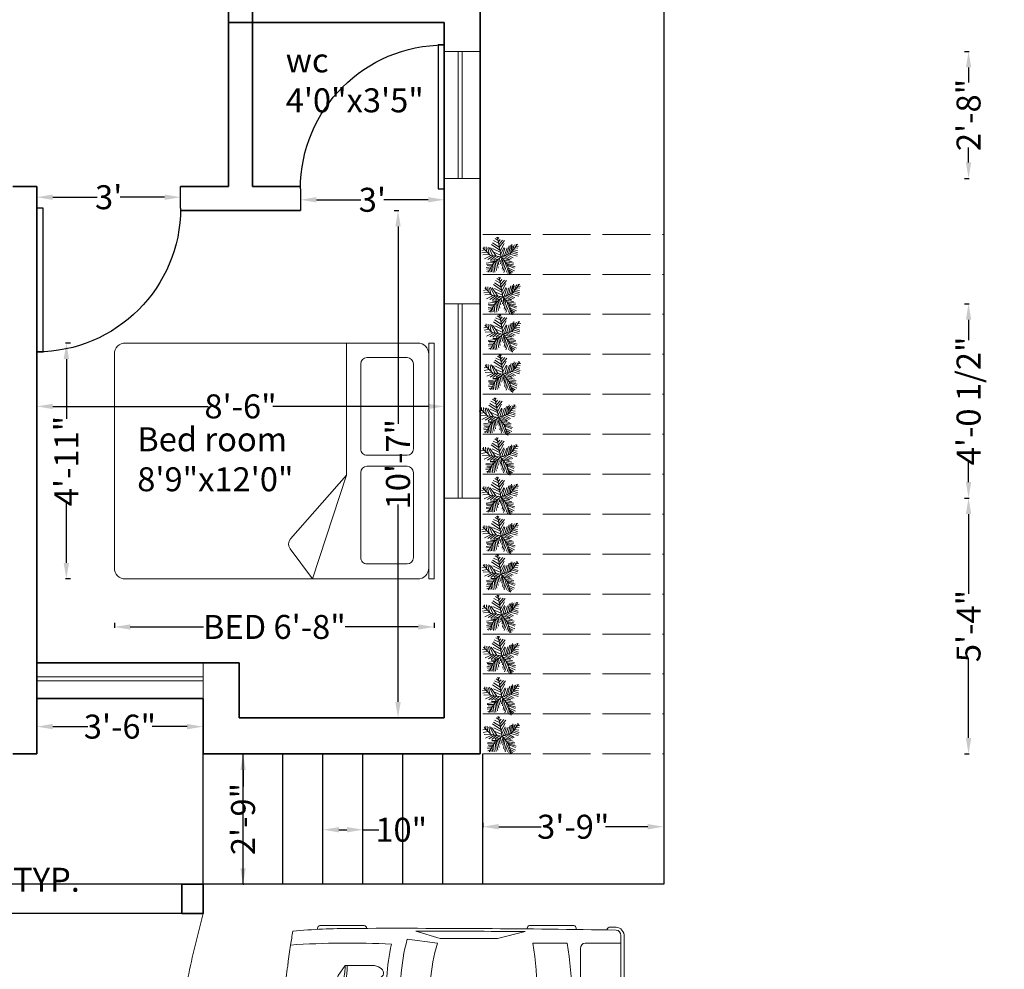
# Model space of a CAD drawing. Units: inches. Extents: x -81 to 380, y -521 to 79.
# Tile 4 of 5: x 134 to 380, y -313 to -76. Entities that reach past the tile are written whole.
import ezdxf

# ---------------------------------------------------------------- set-up
doc = ezdxf.new("R2010")
doc.units = ezdxf.units.IN
doc.header["$MEASUREMENT"] = 0
doc.linetypes.add('ACAD_ISO02W100', pattern=[15, 12, -3])
for name, color, linetype, lineweight in [('A-ANNO-DIMS', 2, 'Continuous', 18), ('A-AREA-IDEN', 5, 'Continuous', 25), ('A-COLS', 34, 'Continuous', 35), ('A-FLOR', 6, 'Continuous', 25), ('A-FLOR-STRS', 6, 'Continuous', 25), ('A-FLOR-STRS-OVHD', 6, 'ACAD_ISO02W100', 18), ('A-FURN', 8, 'Continuous', 18), ('A-GLAZ', 4, 'Continuous', 18), ('A-WALL', 249, 'Continuous', 35), ('C-ROAD-DRWY', 6, 'Continuous', 18), ('car', 33, 'Continuous', 18), ('door', 34, 'Continuous', 25), ('trees', 3, 'Continuous', 13)]:
    doc.layers.add(name, color=color, linetype=linetype, lineweight=lineweight)
doc.styles.get("Standard").update_dxf_attribs({"font": 'arial.ttf'})
doc.dimstyles.get("Standard").update_dxf_attribs({"dimtxt": 6, "dimasz": 4, "dimexe": 0.18, "dimexo": 0.0625, "dimgap": 0.09, "dimtad": 0, "dimdec": 0, "dimzin": 0, "dimdsep": 46, "dimlunit": 3, "dimtxsty": 'Standard', "dimcen": 0.09, "dimclrd": 6, "dimclre": 6, "dimclrt": 2, "dimadec": 0, "dimazin": 0, "dimtfac": 1, "dimtdec": 0, "dimtofl": 0, "dimtmove": 0, "dimatfit": 3, "dimfxl": 1, "dimfxlon": 1, "dimtolj": 1, "dimtzin": 0, "dimarcsym": 0})

# ---------------------------------------------------------------- blocks, each defined once
blk = doc.blocks.new('*U2')
for p, q in [((0, 0), (0, -6)), ((40, 0), (40, -6))]:
    blk.add_line(p, q)
blk.add_lwpolyline([(0, 0), (0, 40), (1.75, 40), (1.75, 0)], close=True)
blk.add_arc((0, 0), 40, 0, 90)
blk = doc.blocks.new('*U4')
for p, q in [((-48.585, 21.131), (-49.309, 29.026)), ((-43.513, 28.561), (-42.427, 15.558)), ((-3.665, 19.273), (-27.574, 35.527)), ((-5.114, 28.097), (-24.676, 40.636)), ((-7.288, 39.707), (-21.778, 46.673)), ((-8.737, 47.138), (-17.069, 52.711)), ((-10.186, 53.64), (-13.084, 55.962)), ((0, 0), (-10.5, 57)), ((-9.099, 51.782), (-6.563, 55.962)), ((-7.65, 43.423), (-2.578, 49.46)), ((-5.839, 35.992), (4.667, 48.067)), ((-5.114, 27.632), (10.463, 46.673)), ((-2.941, 16.486), (8.652, 37.85)), ((16.259, 5.805), (23.142, 31.348)), ((22.055, 7.198), (27.489, 32.277)), ((27, 9), (48, 36)), ((27.127, 9.056), (31.112, 35.992)), ((31.836, 30.883), (32.561, 16.486)), ((35.096, 32.741), (37.27, 22.524)), ((38.719, 34.134), (41.979, 28.561)), ((43.791, 29.954), (51.036, 30.883)), ((44.153, 36.456), (45.239, 32.741)), ((-47.498, 19.737), (-55.83, 18.344)), ((-40.615, 13.7), (-55.105, 10.913)), ((-31.5, 4.5), (-52.5, 25.5)), ((-33.37, 6.269), (-52.207, 5.34)), ((-28.299, 3.483), (-47.86, -5.805)), ((-38.442, 26.239), (-34.819, 7.663)), ((-21.416, 3.018), (-38.079, -8.128)), ((-35.544, 28.097), (-24.314, 3.947)), ((0, 0), (-31.5, 4.5)), ((-14.533, 2.09), (-30.834, 25.31)), ((-15.982, 2.09), (-30.11, -9.521)), ((-24.314, 23.917), (-2.941, 13.7)), ((0, 0), (-22.5, -19.5)), ((-6.563, 1.161), (-21.416, -8.128)), ((-20.691, 13.7), (-1.129, 4.876)), ((-1.129, 6.734), (9.014, 26.704)), ((0, 0), (27, 9)), ((0, 0), (18, -22.5)), ((3.942, 1.625), (11.187, 24.381)), ((6.478, 1.625), (26.04, -8.592)), ((10.101, 3.483), (17.708, 26.239)), ((11.187, 3.483), (30.749, -5.805)), ((18.07, 5.805), (35.096, -3.483)), ((24.229, 7.663), (46.688, 1.625)), ((29.662, 12.307), (48.137, 6.269)), ((33.285, 16.486), (48.862, 10.913)), ((36.183, 19.737), (48.137, 17.88)), ((40.53, 25.775), (48.862, 24.846)), ((-17.431, -15.094), (-42.789, -18.809)), ((-24.314, -21.596), (-42.427, -22.06)), ((-26.849, -26.24), (-40.253, -25.775)), ((-22.5, -19.5), (-37.5, -45)), ((-15.257, -12.772), (-30.11, -12.772)), ((-25.038, -23.918), (-22.865, -45.281)), ((-20.691, -18.345), (-17.793, -44.352)), ((-6.563, -5.805), (-19.967, -9.985)), ((-17.069, -15.094), (-12.721, -40.172)), ((-13.446, -11.378), (-8.737, -32.741)), ((-9.461, -8.592), (-6.201, -23.453)), ((-4.752, -3.483), (-3.665, -14.629)), ((2.493, -3.019), (-1.491, -20.202)), ((1.769, -2.555), (24.229, -9.521)), ((5.029, -6.27), (2.131, -25.775)), ((9.014, -11.378), (3.58, -35.992)), ((14.085, -16.951), (6.478, -40.172)), ((7.565, -9.056), (32.198, -14.629)), ((18.07, -22.524), (8.289, -45.745)), ((12.274, -15.094), (36.907, -18.809)), ((16.259, -19.738), (36.183, -22.989)), ((18, -22.5), (27, -52.5)), ((18.433, -22.524), (40.53, -29.026)), ((19.157, -25.311), (38.719, -33.206)), ((-28.299, -29.026), (-42.789, -31.348)), ((-30.834, -34.135), (-42.427, -35.528)), ((-34.457, -39.708), (-40.978, -42.494)), ((-32.646, -36.921), (-31.921, -44.352)), ((-29.023, -30.884), (-27.936, -43.887)), ((20.244, -30.419), (15.897, -44.816)), ((22.78, -37.85), (19.519, -48.532)), ((21.331, -32.741), (39.081, -40.636)), ((22.78, -38.314), (34.372, -44.816)), ((24.591, -45.745), (23.142, -50.854)), ((24.591, -43.423), (30.749, -47.603)), ((26.764, -49.925), (28.213, -50.854))]:
    blk.add_line(p, q)
blk = doc.blocks.new('*D10')
at = {"layer": 'A-ANNO-DIMS', "color": 0, "lineweight": -2, "transparency": 16777216}
for p, q in [((249.94, -276.74), (249.94, -277.92)), ((253.94, -277.74), (264.52, -277.74)), ((291.22, -277.74), (280.64, -277.74)), ((295.22, -276.74), (295.22, -277.92))]:
    blk.add_line(p, q, dxfattribs=at)
at = {"layer": 'A-ANNO-DIMS', "color": 0, "transparency": 16777216}
for points in [[(253.94, -277.07), (253.94, -278.41), (249.94, -277.74)], [(291.22, -277.07), (291.22, -278.41), (295.22, -277.74)]]:
    blk.add_solid(points, dxfattribs=at)
at = {"layer": 'Defpoints', "color": 0, "transparency": 16777216}
for p in [(249.94, -275.81), (295.22, -275.81), (295.22, -277.74)]:
    blk.add_point(p, dxfattribs=at)
at = {"layer": 'A-ANNO-DIMS', "color": 0, "transparency": 16777216, "insert": (272.58, -277.74), "char_height": 6, "attachment_point": 5}
blk.add_mtext('\\A1;3\'-9"', dxfattribs=at)
blk = doc.blocks.new('*D19')
at = {"layer": 'A-ANNO-DIMS', "color": 0, "lineweight": -2, "transparency": 16777216}
for p, q in [((227.73, -123.52), (228.91, -123.52)), ((228.73, -127.52), (228.73, -176.91)), ((228.73, -246.52), (228.73, -197.13)), ((227.73, -250.52), (228.91, -250.52))]:
    blk.add_line(p, q, dxfattribs=at)
at = {"layer": 'A-ANNO-DIMS', "color": 0, "transparency": 16777216}
for points in [[(228.06, -127.52), (229.4, -127.52), (228.73, -123.52)], [(228.06, -246.52), (229.4, -246.52), (228.73, -250.52)]]:
    blk.add_solid(points, dxfattribs=at)
at = {"layer": 'Defpoints', "color": 0, "transparency": 16777216}
for p in [(200.31, -123.52), (200.31, -250.52), (228.73, -250.52)]:
    blk.add_point(p, dxfattribs=at)
at = {"layer": 'A-ANNO-DIMS', "color": 0, "transparency": 16777216, "insert": (228.73, -187.02), "char_height": 6, "attachment_point": 5, "rotation": 90}
blk.add_mtext('\\A1;10\'-7"', dxfattribs=at)
blk = doc.blocks.new('*D20')
at = {"layer": 'A-ANNO-DIMS', "color": 0, "lineweight": -2, "transparency": 16777216}
for p, q in [((138.31, -172.56), (138.31, -172.38)), ((240.31, -172.56), (240.31, -172.38)), ((142.31, -172.56), (181.24, -172.56)), ((236.31, -172.56), (197.38, -172.56))]:
    blk.add_line(p, q, dxfattribs=at)
at = {"layer": 'A-ANNO-DIMS', "color": 0, "transparency": 16777216}
for points in [[(142.31, -171.9), (142.31, -173.23), (138.31, -172.56)], [(236.31, -171.9), (236.31, -173.23), (240.31, -172.56)]]:
    blk.add_solid(points, dxfattribs=at)
at = {"layer": 'Defpoints', "color": 0, "transparency": 16777216}
for p in [(138.31, -172.56), (240.31, -172.56), (240.31, -172.56)]:
    blk.add_point(p, dxfattribs=at)
at = {"layer": 'A-ANNO-DIMS', "color": 0, "transparency": 16777216, "insert": (189.31, -172.56), "char_height": 6, "attachment_point": 5}
blk.add_mtext('\\A1;8\'-6"', dxfattribs=at)
blk = doc.blocks.new('*D24')
at = {"layer": 'A-ANNO-DIMS', "color": 0, "lineweight": -2, "transparency": 16777216}
for p, q in [((138.31, -120.22), (138.31, -120.04)), ((142.31, -120.22), (153.46, -120.22)), ((170.31, -120.22), (159.16, -120.22)), ((174.31, -120.22), (174.31, -120.04))]:
    blk.add_line(p, q, dxfattribs=at)
at = {"layer": 'A-ANNO-DIMS', "color": 0, "transparency": 16777216}
for points in [[(142.31, -119.55), (142.31, -120.89), (138.31, -120.22)], [(170.31, -119.55), (170.31, -120.89), (174.31, -120.22)]]:
    blk.add_solid(points, dxfattribs=at)
at = {"layer": 'Defpoints', "color": 0, "transparency": 16777216}
for p in [(138.31, -120.22), (174.31, -120.22), (174.31, -120.22)]:
    blk.add_point(p, dxfattribs=at)
at = {"layer": 'A-ANNO-DIMS', "color": 0, "transparency": 16777216, "insert": (156.31, -120.22), "char_height": 6, "attachment_point": 5}
blk.add_mtext("\\A1;3'", dxfattribs=at)
blk = doc.blocks.new('*D25')
at = {"layer": 'A-ANNO-DIMS', "color": 0, "lineweight": -2, "transparency": 16777216}
for p, q in [((204.31, -120.86), (204.31, -121.04)), ((208.31, -120.86), (219.46, -120.86)), ((236.31, -120.86), (225.16, -120.86)), ((240.31, -120.86), (240.31, -121.04))]:
    blk.add_line(p, q, dxfattribs=at)
at = {"layer": 'A-ANNO-DIMS', "color": 0, "transparency": 16777216}
for points in [[(208.31, -120.19), (208.31, -121.53), (204.31, -120.86)], [(236.31, -120.19), (236.31, -121.53), (240.31, -120.86)]]:
    blk.add_solid(points, dxfattribs=at)
at = {"layer": 'Defpoints', "color": 0, "transparency": 16777216}
for p in [(204.31, -120.82), (240.31, -120.82), (240.31, -120.86)]:
    blk.add_point(p, dxfattribs=at)
at = {"layer": 'A-ANNO-DIMS', "color": 0, "transparency": 16777216, "insert": (222.31, -120.86), "char_height": 6, "attachment_point": 5}
blk.add_mtext("\\A1;3'", dxfattribs=at)
blk = doc.blocks.new('*D29')
at = {"layer": 'A-ANNO-DIMS', "color": 0, "lineweight": -2, "transparency": 16777216}
for p, q in [((138.31, -252.67), (138.31, -252.87)), ((142.31, -252.69), (151.07, -252.69)), ((175.94, -252.69), (167.19, -252.69)), ((179.94, -252.67), (179.94, -252.87))]:
    blk.add_line(p, q, dxfattribs=at)
at = {"layer": 'A-ANNO-DIMS', "color": 0, "transparency": 16777216}
for points in [[(142.31, -252.02), (142.31, -253.36), (138.31, -252.69)], [(175.94, -252.02), (175.94, -253.36), (179.94, -252.69)]]:
    blk.add_solid(points, dxfattribs=at)
at = {"layer": 'Defpoints', "color": 0, "transparency": 16777216}
for p in [(138.31, -252.6), (138.31, -252.69), (179.94, -252.6)]:
    blk.add_point(p, dxfattribs=at)
at = {"layer": 'A-ANNO-DIMS', "color": 0, "transparency": 16777216, "insert": (159.13, -252.69), "char_height": 6, "attachment_point": 5}
blk.add_mtext('\\A1;3\'-6"', dxfattribs=at)
blk = doc.blocks.new('*D30')
at = {"layer": 'A-ANNO-DIMS', "color": 0, "lineweight": -2, "transparency": 16777216}
for p, q in [((189.94, -259.52), (190.12, -259.52)), ((189.94, -263.52), (189.94, -267.7)), ((189.94, -288.11), (189.94, -283.93)), ((189.94, -292.11), (190.12, -292.11))]:
    blk.add_line(p, q, dxfattribs=at)
at = {"layer": 'A-ANNO-DIMS', "color": 0, "transparency": 16777216}
for points in [[(189.28, -263.52), (190.61, -263.52), (189.94, -259.52)], [(189.28, -288.11), (190.61, -288.11), (189.94, -292.11)]]:
    blk.add_solid(points, dxfattribs=at)
at = {"layer": 'Defpoints', "color": 0, "transparency": 16777216}
for p in [(189.94, -259.52), (189.94, -259.52), (189.94, -292.11)]:
    blk.add_point(p, dxfattribs=at)
at = {"layer": 'A-ANNO-DIMS', "color": 0, "transparency": 16777216, "insert": (189.94, -275.81), "char_height": 6, "attachment_point": 5, "rotation": 90}
blk.add_mtext('\\A1;2\'-9"', dxfattribs=at)
blk = doc.blocks.new('*D31')
at = {"layer": 'A-ANNO-DIMS', "color": 0, "lineweight": -2, "transparency": 16777216}
for p, q in [((209.94, -278.49), (209.94, -278.31)), ((219.94, -278.49), (219.94, -278.31)), ((213.94, -278.49), (215.94, -278.49)), ((219.94, -278.49), (223.94, -278.49))]:
    blk.add_line(p, q, dxfattribs=at)
at = {"layer": 'A-ANNO-DIMS', "color": 0, "transparency": 16777216}
for points in [[(213.94, -277.82), (213.94, -279.15), (209.94, -278.49)], [(215.94, -277.82), (215.94, -279.15), (219.94, -278.49)]]:
    blk.add_solid(points, dxfattribs=at)
at = {"layer": 'Defpoints', "color": 0, "transparency": 16777216}
for p in [(209.94, -278.49), (219.94, -278.49), (219.94, -278.49)]:
    blk.add_point(p, dxfattribs=at)
at = {"layer": 'A-ANNO-DIMS', "color": 0, "transparency": 16777216, "insert": (229.53, -278.49), "char_height": 6, "attachment_point": 5}
blk.add_mtext('\\A1;10"', dxfattribs=at)
blk = doc.blocks.new('*U33')
for p, q in [((46.55, 38.89), (22.35, 38.89)), ((136.7, 38.89), (160.9, 38.89)), ((21.1, 37.41), (21.1, 36.83)), ((47.8, 37.39), (47.8, 37.41)), ((87.99, 31.87), (74.76, 35.92)), ((134.31, 35.6), (119.29, 31.78)), ((135.45, 37.07), (135.45, 37.41)), ((162.15, 37.41), (162.15, 36.77)), ((186.47, -33.5), (186.47, 33.5)), ((188.4, -32.76), (188.4, 32.76)), ((70.03, 31.54), (86.41, 29.35)), ((138.42, 29.35), (157.25, 29.35)), ((186.47, 29.35), (167.01, 29.35)), ((164.52, 26.39), (164.52, -26.39)), ((32.27, 11.63), (36.13, 17.17)), ((36.13, 17.17), (50.94, 17.17)), ((32.12, 9.51), (32.12, 11.15)), ((58.92, -10.77), (58.92, 10.77)), ((3.27, 6.13), (0.1, 0.41)), ((29.77, 9.51), (51.68, 9.51)), ((66.55, -10.53), (66.55, 10.53)), ((82.74, 8.5), (82.74, -8.5)), ((186.47, -10.53), (186.47, 10.53)), ((0, 0), (51.68, 0)), ((0.1, -0.41), (3.27, -6.13)), ((29.77, -9.51), (51.68, -9.51)), ((32.12, -9.51), (32.12, -11.15)), ((32.27, -11.63), (36.13, -17.17)), ((36.13, -17.17), (50.94, -17.17)), ((86.41, -29.35), (70.03, -31.54)), ((87.99, -31.87), (74.76, -35.92)), ((134.31, -35.6), (119.29, -31.78)), ((157.25, -29.35), (138.42, -29.35)), ((167.01, -29.35), (186.47, -29.35)), ((21.1, -37.41), (21.1, -36.83)), ((47.8, -37.39), (47.8, -37.41)), ((135.45, -37.07), (135.45, -37.41)), ((162.15, -37.41), (162.15, -36.77)), ((46.55, -38.89), (22.35, -38.89)), ((136.7, -38.89), (160.9, -38.89))]:
    blk.add_line(p, q)
for centre, major_axis, ratio, start_param, end_param in [((22.35, 37.41), (0, -1.48), 0.842304, 3.141593, 4.712389), ((46.55, 37.41), (0, 1.48), 0.842304, -1.570796, 0), ((136.7, 37.41), (0, -1.48), 0.842304, 3.141593, 4.712389), ((160.9, 37.41), (0, 1.48), 0.842304, -1.570796, 0), ((180.63, 35.84), (0, 2.22), 0.842304, -0.013017, 1.249894), ((64.48, -10556.36), (0, 10595.31), 0.842304, -0.013397, -0.013017), ((183.98, 32.76), (0, -5.25), 0.842304, 1.570796, 3.128196), ((266.03, -27.52), (0, 313.31), 0.842304, 1.367076, 1.39176), ((41.19, -490.86), (0, 528.23), 0.842304, 0.00281, 0.075598), ((64.48, -10555.62), (0, 10593.03), 0.842304, -0.013397, 0.002797), ((64.48, -10555.62), (0, -10591.55), 0.842304, 3.133765, 3.140441), ((183.98, 33.5), (0, -2.96), 0.842304, 1.570796, 3.128196), ((259.18, -27.52), (0, -305.3), 0.842304, 4.528606, 4.561838), ((37.47, -593.96), (0, -623.33), 0.842304, 3.096046, 3.200911), ((134.4, 5.39), (0, -89.78), 0.842304, 4.449482, 4.652344), ((135.29, 5.39), (0, 81.77), 0.842304, 1.245306, 1.50788), ((149.6, 2.8), (0, -79.58), 0.842304, 4.372215, 4.640744), ((95.79, -3666.35), (0, -3698.24), 0.842304, 3.134049, 3.144098), ((17.08, 0), (0, 147.02), 0.842304, 4.511394, 4.913384), ((35.91, 0), (0, 147.02), 0.842304, 4.511394, 4.913384), ((167.01, 26.39), (0, 2.96), 0.842304, 0, 1.570796), ((-204.49, 52.4), (0, -250.96), 0.842304, 1.385369, 1.434372), ((13.04, 17.01), (0, 27.42), 0.842304, 4.435146, 4.718221), ((14.2, 17.01), (0, 27.42), 0.842304, 4.435146, 4.718221), ((50.79, 13.34), (6.34, -0.36), 0.603834, -1.395552, 1.581315), ((32.75, 11.15), (0, 0.74), 0.842304, 0.879714, 1.570796), ((29.77, -46.66), (0, 56.17), 0.842304, 0, 0.590319), ((0.62, 0), (0, -0.74), 0.842304, 4.131459, 5.293319), ((29.77, 46.66), (0, 56.17), 0.842304, 2.551274, 3.141593), ((-204.49, -52.4), (0, 250.96), 0.842304, -1.434372, -1.385369), ((13.04, -17.01), (0, -27.42), 0.842304, 1.564964, 1.848039), ((14.2, -17.01), (0, -27.42), 0.842304, 1.564964, 1.848039), ((135.29, -5.39), (0, -81.77), 0.842304, -1.50788, -1.245306), ((149.6, -2.8), (0, -79.58), 0.842304, -1.499151, -1.230623), ((32.75, -11.15), (0, -0.74), 0.842304, 4.712389, 5.403472), ((134.4, -5.39), (0, -89.78), 0.842304, -1.510751, -1.307889), ((259.18, 27.52), (0, 305.3), 0.842304, 1.721348, 1.754579), ((167.01, -26.39), (0, -2.96), 0.842304, 4.712389, 6.283185), ((266.03, 27.52), (0, 313.31), 0.842304, 1.749832, 1.774517), ((37.47, 593.96), (0, -623.33), 0.842304, -0.059319, 0.045547), ((95.79, 3666.35), (0, -3698.24), 0.842304, -0.002505, 0.007544), ((41.19, 490.86), (0, -528.23), 0.842304, -0.075598, -0.00281), ((22.35, -37.41), (0, 1.48), 0.842304, 1.570796, 3.141593), ((64.48, 10555.62), (0, 10593.03), 0.842304, 3.138796, 3.15499), ((46.55, -37.41), (0, -1.48), 0.842304, 0, 1.570796), ((64.48, 10555.62), (0, -10591.55), 0.842304, 0.001152, 0.007828), ((136.7, -37.41), (0, -1.48), 0.842304, -1.570796, 0), ((160.9, -37.41), (0, 1.48), 0.842304, 3.141593, 4.712389), ((180.63, -35.84), (0, -2.22), 0.842304, -1.249894, 0.013017), ((183.98, -33.5), (0, 2.96), 0.842304, 3.15499, 4.712389), ((183.98, -32.76), (0, -5.25), 0.842304, 0.013397, 1.570796), ((64.48, 10556.36), (0, 10595.31), 0.842304, 3.15461, 3.15499)]:
    blk.add_ellipse(centre, major_axis=major_axis, ratio=ratio, start_param=start_param, end_param=end_param)
at = {"extrusion": (0, 0, -1)}
blk.add_ellipse((50.79, -13.34), major_axis=(6.34, 0.36), ratio=0.603834, start_param=-1.395552, end_param=1.581315, dxfattribs=at)
blk = doc.blocks.new('A$C164346CA')
for p, q in [((0, 2.035), (0, 2)), ((1.5, 2.035), (0, 2.035)), ((1.5, 2), (1.5, 2.035)), ((1.5, 2), (0, 2)), ((0, 1.93), (0, 0.07)), ((0.6731, 1.9024), (0.1319, 1.9024)), ((1.364, 1.9024), (0.8228, 1.9024)), ((1.5, 0.07), (1.5, 1.93)), ((0.0919, 1.8624), (0.0919, 1.6069)), ((0.7131, 1.6069), (0.7131, 1.8624)), ((0.7828, 1.8624), (0.7828, 1.6069)), ((1.404, 1.6069), (1.404, 1.8624)), ((0.1319, 1.5669), (0.6731, 1.5669)), ((0.8228, 1.5669), (1.364, 1.5669)), ((0.8395, 1.4761), (0, 1.4761)), ((0.8395, 1.4761), (1.2448, 1.12)), ((1.5, 1.2611), (0.8395, 1.4761)), ((1.3077, 1.1175), (1.5, 1.2611)), ((0.07, 0), (1.43, 0))]:
    blk.add_line(p, q)
for centre, radius, start, end in [((0.07, 1.93), 0.07, 90, 180), ((1.43, 1.93), 0.07, 0, 90), ((0.1319, 1.8624), 0.04, 90, 180), ((0.6731, 1.8624), 0.04, 0, 90), ((0.8228, 1.8624), 0.04, 90, 180), ((1.364, 1.8624), 0.04, 0, 90), ((0.1319, 1.6069), 0.04, 180, 270), ((0.6731, 1.6069), 0.04, 270, 0), ((0.8228, 1.6069), 0.04, 180, 270), ((1.364, 1.6069), 0.04, 270, 0), ((1.2778, 1.1575), 0.05, 228.69584, 306.75789), ((0.07, 0.07), 0.07, 180, 270), ((1.43, 0.07), 0.07, 270, 0)]:
    blk.add_arc(centre, radius, start, end)
blk = doc.blocks.new('ENTRY-POST')
blk.add_lwpolyline([(0, 7.31), (5.28, 7.31), (5.28, 0), (0, 0)], close=True)
blk = doc.blocks.new('*D39')
at = {"layer": 'A-ANNO-DIMS', "color": 6, "lineweight": -2, "transparency": 16777216}
for p, q in [((81.08, -291.01), (77.08, -291.01)), ((85.08, -292.01), (85.08, -290.83)), ((90.37, -292.01), (90.37, -290.83)), ((94.37, -291.01), (98.37, -291.01))]:
    blk.add_line(p, q, dxfattribs=at)
at = {"layer": 'A-ANNO-DIMS', "color": 6, "transparency": 16777216}
for points in [[(81.08, -290.34), (81.08, -291.68), (85.08, -291.01)], [(94.37, -290.34), (94.37, -291.68), (90.37, -291.01)]]:
    blk.add_solid(points, dxfattribs=at)
at = {"layer": 'Defpoints', "color": 0, "transparency": 16777216}
for p in [(85.08, -292.11), (90.37, -291.01), (90.37, -292.11)]:
    blk.add_point(p, dxfattribs=at)
at = {"layer": 'A-ANNO-DIMS', "color": 2, "transparency": 16777216, "insert": (123.73, -291.01), "char_height": 6, "attachment_point": 5}
blk.add_mtext('\\A1;0\'-5 1/2" TYP.', dxfattribs=at)
blk = doc.blocks.new('*D40')
at = {"layer": 'A-ANNO-DIMS', "color": 6, "lineweight": -2, "transparency": 16777216}
for p, q in [((157.73, -226.75), (157.73, -227.93)), ((161.73, -227.75), (180.05, -227.75)), ((233.8, -227.75), (215.48, -227.75)), ((237.8, -226.75), (237.8, -227.93))]:
    blk.add_line(p, q, dxfattribs=at)
at = {"layer": 'A-ANNO-DIMS', "color": 6, "transparency": 16777216}
for points in [[(161.73, -227.09), (161.73, -228.42), (157.73, -227.75)], [(233.8, -227.09), (233.8, -228.42), (237.8, -227.75)]]:
    blk.add_solid(points, dxfattribs=at)
at = {"layer": 'Defpoints', "color": 0, "transparency": 16777216}
for p in [(157.73, -215.74), (237.8, -215.74), (237.8, -227.75)]:
    blk.add_point(p, dxfattribs=at)
at = {"layer": 'A-ANNO-DIMS', "color": 2, "transparency": 16777216, "insert": (197.77, -227.75), "char_height": 6, "attachment_point": 5}
blk.add_mtext('\\A1;BED 6\'-8"', dxfattribs=at)
blk = doc.blocks.new('*D41')
at = {"layer": 'A-ANNO-DIMS', "color": 6, "lineweight": -2, "transparency": 16777216}
for p, q in [((146.72, -156.72), (145.54, -156.72)), ((145.72, -160.72), (145.72, -175.71)), ((145.72, -211.74), (145.72, -196.75)), ((146.72, -215.74), (145.54, -215.74))]:
    blk.add_line(p, q, dxfattribs=at)
at = {"layer": 'A-ANNO-DIMS', "color": 6, "transparency": 16777216}
for points in [[(145.05, -160.72), (146.38, -160.72), (145.72, -156.72)], [(145.05, -211.74), (146.38, -211.74), (145.72, -215.74)]]:
    blk.add_solid(points, dxfattribs=at)
at = {"layer": 'Defpoints', "color": 0, "transparency": 16777216}
for p in [(157.73, -156.72), (145.72, -215.74), (157.73, -215.74)]:
    blk.add_point(p, dxfattribs=at)
at = {"layer": 'A-ANNO-DIMS', "color": 2, "transparency": 16777216, "insert": (145.72, -186.23), "char_height": 6, "attachment_point": 5, "rotation": 90}
blk.add_mtext('\\A1;4\'-11"', dxfattribs=at)
blk = doc.blocks.new('*D46')
at = {"layer": 'A-ANNO-DIMS', "color": 6, "lineweight": -2, "transparency": 16777216}
for p, q in [((74.55, 54.93), (74.55, 56.11)), ((78.55, 55.93), (124.45, 55.93)), ((186.48, 55.93), (140.58, 55.93)), ((190.48, 54.93), (190.48, 56.11))]:
    blk.add_line(p, q, dxfattribs=at)
at = {"layer": 'A-ANNO-DIMS', "color": 6, "transparency": 16777216}
for points in [[(78.55, 56.6), (78.55, 55.26), (74.55, 55.93)], [(186.48, 56.6), (186.48, 55.26), (190.48, 55.93)]]:
    blk.add_solid(points, dxfattribs=at)
at = {"layer": 'Defpoints', "color": 0, "transparency": 16777216}
for p in [(190.48, 55.93), (74.55, -489.67), (190.48, -489.67)]:
    blk.add_point(p, dxfattribs=at)
at = {"layer": 'A-ANNO-DIMS', "color": 2, "transparency": 16777216, "insert": (132.51, 55.93), "char_height": 6, "attachment_point": 5}
blk.add_mtext('\\A1;9\'-8"', dxfattribs=at)
blk = doc.blocks.new('*D49')
at = {"layer": 'A-ANNO-DIMS', "color": 6, "lineweight": -2, "transparency": 16777216}
for p, q in [((85.08, -516.12), (85.08, -517.3)), ((89.08, -517.12), (122.14, -517.12)), ((175.94, -517.12), (142.88, -517.12)), ((179.94, -516.12), (179.94, -517.3))]:
    blk.add_line(p, q, dxfattribs=at)
at = {"layer": 'A-ANNO-DIMS', "color": 6, "transparency": 16777216}
for points in [[(89.08, -516.45), (89.08, -517.79), (85.08, -517.12)], [(175.94, -516.45), (175.94, -517.79), (179.94, -517.12)]]:
    blk.add_solid(points, dxfattribs=at)
at = {"layer": 'Defpoints', "color": 0, "transparency": 16777216}
for p in [(85.08, -299.41), (179.94, -299.41), (179.94, -517.12)]:
    blk.add_point(p, dxfattribs=at)
at = {"layer": 'A-ANNO-DIMS', "color": 2, "transparency": 16777216, "insert": (132.51, -517.12), "char_height": 6, "attachment_point": 5}
blk.add_mtext('\\A1;7\'-11"', dxfattribs=at)
blk = doc.blocks.new('*D52')
at = {"layer": 'A-ANNO-DIMS', "color": 6, "lineweight": -2, "transparency": 16777216}
for p, q in [((179.94, -516.12), (179.94, -517.3)), ((183.94, -517.12), (204.55, -517.12)), ((245.94, -517.12), (225.34, -517.12)), ((249.94, -516.12), (249.94, -517.3))]:
    blk.add_line(p, q, dxfattribs=at)
at = {"layer": 'A-ANNO-DIMS', "color": 6, "transparency": 16777216}
for points in [[(183.94, -516.45), (183.94, -517.79), (179.94, -517.12)], [(245.94, -516.45), (245.94, -517.79), (249.94, -517.12)]]:
    blk.add_solid(points, dxfattribs=at)
at = {"layer": 'Defpoints', "color": 0, "transparency": 16777216}
for p in [(179.94, -292.11), (249.94, -292.11), (249.94, -517.12)]:
    blk.add_point(p, dxfattribs=at)
at = {"layer": 'A-ANNO-DIMS', "color": 2, "transparency": 16777216, "insert": (214.94, -517.12), "char_height": 6, "attachment_point": 5}
blk.add_mtext('\\A1;5\'-10"', dxfattribs=at)
blk = doc.blocks.new('*D64')
at = {"layer": 'A-ANNO-DIMS', "color": 6, "lineweight": -2, "transparency": 16777216}
for p, q in [((370.52, -146.87), (371.7, -146.87)), ((371.52, -150.87), (371.52, -156.01)), ((371.52, -191.49), (371.52, -186.36)), ((370.52, -195.49), (371.7, -195.49))]:
    blk.add_line(p, q, dxfattribs=at)
at = {"layer": 'A-ANNO-DIMS', "color": 6, "transparency": 16777216}
for points in [[(370.86, -150.87), (372.19, -150.87), (371.52, -146.87)], [(370.86, -191.49), (372.19, -191.49), (371.52, -195.49)]]:
    blk.add_solid(points, dxfattribs=at)
at = {"layer": 'Defpoints', "color": 0, "transparency": 16777216}
for p in [(249.31, -146.87), (371.52, -146.87), (249.31, -195.49)]:
    blk.add_point(p, dxfattribs=at)
at = {"layer": 'A-ANNO-DIMS', "color": 2, "transparency": 16777216, "insert": (371.52, -171.18), "char_height": 6, "attachment_point": 5, "rotation": 90}
blk.add_mtext('\\A1;4\'-0 1/2"', dxfattribs=at)
blk = doc.blocks.new('*D65')
at = {"layer": 'A-ANNO-DIMS', "color": 6, "lineweight": -2, "transparency": 16777216}
for p, q in [((370.52, -195.49), (371.7, -195.49)), ((371.52, -199.49), (371.52, -219.44)), ((371.52, -255.52), (371.52, -235.57)), ((370.52, -259.52), (371.7, -259.52))]:
    blk.add_line(p, q, dxfattribs=at)
at = {"layer": 'A-ANNO-DIMS', "color": 6, "transparency": 16777216}
for points in [[(370.86, -199.49), (372.19, -199.49), (371.52, -195.49)], [(370.86, -255.52), (372.19, -255.52), (371.52, -259.52)]]:
    blk.add_solid(points, dxfattribs=at)
at = {"layer": 'Defpoints', "color": 0, "transparency": 16777216}
for p in [(249.31, -195.49), (249.31, -259.52), (371.52, -259.52)]:
    blk.add_point(p, dxfattribs=at)
at = {"layer": 'A-ANNO-DIMS', "color": 2, "transparency": 16777216, "insert": (371.52, -227.51), "char_height": 6, "attachment_point": 5, "rotation": 90}
blk.add_mtext('\\A1;5\'-4"', dxfattribs=at)
blk = doc.blocks.new('*D66')
at = {"layer": 'A-ANNO-DIMS', "color": 6, "lineweight": -2, "transparency": 16777216}
for p, q in [((370.52, -83.75), (371.7, -83.75)), ((371.52, -87.75), (371.52, -91.52)), ((371.52, -111.52), (371.52, -107.75)), ((370.52, -115.52), (371.7, -115.52))]:
    blk.add_line(p, q, dxfattribs=at)
at = {"layer": 'A-ANNO-DIMS', "color": 6, "transparency": 16777216}
for points in [[(370.86, -87.75), (372.19, -87.75), (371.52, -83.75)], [(370.86, -111.52), (372.19, -111.52), (371.52, -115.52)]]:
    blk.add_solid(points, dxfattribs=at)
at = {"layer": 'Defpoints', "color": 0, "transparency": 16777216}
for p in [(249.31, -83.75), (371.52, -83.75), (249.31, -115.52)]:
    blk.add_point(p, dxfattribs=at)
at = {"layer": 'A-ANNO-DIMS', "color": 2, "transparency": 16777216, "insert": (371.52, -99.63), "char_height": 6, "attachment_point": 5, "rotation": 90}
blk.add_mtext('\\A1;2\'-8"', dxfattribs=at)

msp = doc.modelspace()

# ---------------------------------------------------------------- linework, layer by layer
at = {"layer": 'A-FLOR'}
for p, q in [((179.94, -292.11), (85.08, -292.11)), ((179.94, -299.41), (85.08, -299.41))]:
    msp.add_line(p, q, dxfattribs=at)
at = {"layer": 'A-FLOR-STRS'}
for p, q in [((295.22, -52.91), (295.22, -292.11)), ((179.94, -292.11), (179.94, -259.52)), ((189.94, -292.11), (189.94, -259.52)), ((199.94, -292.11), (199.94, -259.52)), ((209.94, -292.11), (209.94, -259.52)), ((219.94, -292.11), (219.94, -259.52)), ((229.94, -292.11), (229.94, -259.52)), ((239.94, -292.11), (239.94, -259.52)), ((249.94, -292.11), (249.94, -259.52)), ((295.22, -292.11), (179.94, -292.11))]:
    msp.add_line(p, q, dxfattribs=at)
at = {"layer": 'A-FLOR-STRS-OVHD'}
for p, q in [((249.94, -129.52), (295.22, -129.52)), ((249.94, -139.52), (295.22, -139.52)), ((249.94, -149.52), (295.22, -149.52)), ((249.94, -159.52), (295.22, -159.52)), ((249.94, -169.52), (295.22, -169.52)), ((249.94, -179.52), (295.22, -179.52)), ((249.94, -189.52), (295.22, -189.52)), ((249.94, -199.52), (295.22, -199.52)), ((249.94, -209.52), (295.22, -209.52)), ((249.94, -219.52), (295.22, -219.52)), ((249.94, -229.52), (295.22, -229.52)), ((249.94, -239.52), (295.22, -239.52)), ((249.94, -249.52), (295.22, -249.52)), ((249.94, -259.52), (295.22, -259.52))]:
    msp.add_line(p, q, dxfattribs=at)
at = {"layer": 'A-GLAZ'}
for p, q in [((240.31, -83.75), (249.31, -83.75)), ((243.81, -115.52), (243.81, -83.75)), ((244.81, -115.52), (244.81, -83.75)), ((240.31, -115.52), (249.31, -115.52)), ((240.31, -146.87), (249.31, -146.87)), ((243.81, -195.49), (243.81, -146.87)), ((244.81, -195.49), (244.81, -146.87)), ((240.31, -195.49), (249.31, -195.49)), ((179.94, -245.69), (179.94, -236.69)), ((179.94, -240.19), (138.31, -240.19)), ((179.94, -241.19), (138.31, -241.19))]:
    msp.add_line(p, q, dxfattribs=at)
at = {"layer": 'A-WALL'}
for p, q in [((249.31, 28.48), (249.31, -259.52)), ((186.31, -70.52), (186.31, -117.52)), ((192.31, -70.52), (192.31, -117.52)), ((186.31, -76.52), (240.31, -76.52)), ((240.31, -76.52), (240.31, -250.52)), ((132.31, -117.52), (138.31, -117.52)), ((138.31, -117.52), (138.31, -250.52)), ((174.31, -117.52), (186.31, -117.52)), ((192.31, -117.52), (204.32, -117.52)), ((174.31, -123.52), (204.31, -123.52)), ((188.94, -236.69), (138.31, -236.69)), ((188.94, -250.52), (188.94, -236.69)), ((179.94, -245.69), (138.31, -245.69)), ((179.94, -259.52), (179.94, -245.69)), ((138.31, -250.52), (138.31, -259.52)), ((188.94, -250.52), (240.31, -250.52)), ((138.31, -259.52), (132.31, -259.52)), ((179.94, -259.52), (249.31, -259.52))]:
    msp.add_line(p, q, dxfattribs=at)
at = {"layer": 'C-ROAD-DRWY'}
msp.add_open_spline([(179.94, -299.41), (178.59, -304.77), (172.86, -327.51), (171.08, -372.63), (168.34, -432.53), (183.36, -471.31), (190.48, -489.67)], degree=3, knots=[0, 0, 0, 0, 16.553876, 70.232148, 135.187628, 193.647877, 193.647877, 193.647877, 193.647877], dxfattribs=at)

# ---------------------------------------------------------------- block references
at = {"layer": 'A-COLS'}
msp.add_blockref('ENTRY-POST', (174.66, -299.41), dxfattribs=at)
at = {"layer": 'A-FURN', "xscale": 39.34857056651051, "yscale": 39.34857056651051, "zscale": 39.34857056651051, "rotation": 270}
msp.add_blockref('A$C164346CA', (157.73, -156.72), dxfattribs=at)
at = {"layer": 'car', "xscale": 0.4587568616370848, "yscale": 0.4587568616370848, "zscale": 0.4587568616370848}
msp.add_blockref('*U33', (198.93, -320.32), dxfattribs=at)
at = {"layer": 'door', "xscale": -0.9, "yscale": 0.9, "zscale": 0.9}
msp.add_blockref('*U2', (240.31, -118.12), dxfattribs=at)
at = {"layer": 'door', "xscale": -0.9, "yscale": 0.9, "zscale": 0.9, "rotation": 180}
msp.add_blockref('*U2', (138.31, -122.92), dxfattribs=at)
at = {"layer": 'trees', "xscale": 0.0864443764377546, "yscale": 0.0864443764377546, "zscale": 0.0864443764377546}
for p in [(254.51, -135.11), (254.97, -145.12), (255.02, -154.45), (255.08, -164.51), (253.86, -175.31), (254.4, -185.27), (254.45, -195.15), (254.51, -204.91), (254.54, -214.53), (254.6, -224.7), (254.68, -234.99), (254.73, -245.27), (254.79, -255.08)]:
    msp.add_blockref('*U4', p, dxfattribs=at)

# ---------------------------------------------------------------- texts
at = {"layer": 'A-AREA-IDEN', "char_height": 6, "attachment_point": 1}
for s, insert in [('wc\\P4\'0"x3\'5"', (200.62, -82.97)), ('Bed room\\P8\'9"x12\'0"', (163.46, -177.79))]:
    msp.add_mtext_dynamic_manual_height_columns(s, width=81.6384, gutter_width=1, heights=[0], dxfattribs=dict(at, insert=insert))

# ---------------------------------------------------------------- dimensions: what is measured, and where the dimension line sits
at = {"layer": 'A-ANNO-DIMS'}
for base, p1, p2, override, picture, middle in [((190.48, 55.93), (74.55, -489.67), (190.48, -489.67), {"dimdec": 1, "dimlfac": 1, "dimrnd": 0, "dimzin": 1, "dimdsep": 46, "dimlunit": 4, "dimfrac": 2}, '*D46', (132.51, 55.93)), ((174.31, -120.22), (138.31, -120.22), (174.31, -120.22), {"dimclrd": 0, "dimclre": 0, "dimclrt": 0}, '*D24', (156.31, -120.22)), ((240.31, -120.86), (204.31, -120.82), (240.31, -120.82), {"dimclrd": 0, "dimclre": 0, "dimclrt": 0}, '*D25', (222.31, -120.86)), ((240.31, -172.56), (138.31, -172.56), (240.31, -172.56), {"dimclrd": 0, "dimclre": 0, "dimclrt": 0}, '*D20', (189.31, -172.56)), ((138.31, -252.69), (179.94, -252.6), (138.31, -252.6), {"dimclrd": 0, "dimclre": 0, "dimclrt": 0}, '*D29', (159.13, -252.69)), ((219.94, -278.49), (209.94, -278.49), (219.94, -278.49), {"dimclrd": 0, "dimclre": 0, "dimclrt": 0}, '*D31', (229.53, -278.49)), ((295.22, -277.74), (249.94, -275.81), (295.22, -275.81), {"dimclrd": 0, "dimclre": 0, "dimclrt": 0}, '*D10', (272.58, -277.74)), ((249.94, -517.12), (179.94, -292.11), (249.94, -292.11), {"dimdec": 1, "dimlfac": 1, "dimrnd": 0, "dimzin": 1, "dimdsep": 46, "dimlunit": 4, "dimfrac": 2}, '*D52', (214.94, -517.12)), ((179.94, -517.12), (85.08, -299.41), (179.94, -299.41), {"dimdec": 1, "dimlfac": 1, "dimrnd": 0, "dimzin": 1, "dimdsep": 46, "dimlunit": 4, "dimfrac": 2}, '*D49', (132.51, -517.12))]:
    dim = msp.add_linear_dim(base=base, p1=p1, p2=p2, dimstyle='Standard', override=override, dxfattribs=at)
    dim.commit()
    dim.dimension.update_dxf_attribs({"geometry": picture, "text_midpoint": middle})
for base, p1, p2, angle, override, picture, middle in [((371.52, -83.75), (249.31, -115.52), (249.31, -83.75), 90, {"dimdec": 1, "dimlfac": 1, "dimrnd": 0, "dimzin": 1, "dimdsep": 46, "dimlunit": 4, "dimfrac": 2}, '*D66', (371.52, -99.63)), ((228.73, -250.52), (200.31, -123.52), (200.31, -250.52), 90, {"dimclrd": 0, "dimclre": 0, "dimclrt": 0}, '*D19', (228.73, -187.02)), ((371.52, -146.87), (249.31, -195.49), (249.31, -146.87), 90, {"dimdec": 1, "dimlfac": 1, "dimrnd": 0, "dimzin": 1, "dimdsep": 46, "dimlunit": 4, "dimfrac": 2}, '*D64', (371.52, -171.18)), ((145.72, -215.74), (157.73, -156.72), (157.73, -215.74), 270, {"dimdec": 1, "dimlfac": 1, "dimrnd": 0, "dimzin": 1, "dimdsep": 46, "dimlunit": 4, "dimfrac": 2}, '*D41', (145.72, -186.23)), ((371.52, -259.52), (249.31, -195.49), (249.31, -259.52), 90, {"dimdec": 1, "dimlfac": 1, "dimrnd": 0, "dimzin": 1, "dimdsep": 46, "dimlunit": 4, "dimfrac": 2}, '*D65', (371.52, -227.51)), ((189.94, -259.52), (189.94, -292.11), (189.94, -259.52), 90, {"dimclrd": 0, "dimclre": 0, "dimclrt": 0}, '*D30', (189.94, -275.81))]:
    dim = msp.add_linear_dim(base=base, p1=p1, p2=p2, angle=angle, dimstyle='Standard', override=override, dxfattribs=at)
    dim.commit()
    dim.dimension.update_dxf_attribs({"geometry": picture, "text_midpoint": middle})
for base, p1, p2, text, picture, middle in [((237.8, -227.75), (157.73, -215.74), (237.8, -215.74), 'BED <>', '*D40', (197.77, -227.75)), ((90.37, -291.01), (85.08, -292.11), (90.37, -292.11), '<> TYP.', '*D39', (123.73, -291.01))]:
    dim = msp.add_linear_dim(base=base, p1=p1, p2=p2, text=text, dimstyle='Standard', override={"dimdec": 1, "dimlfac": 1, "dimrnd": 0, "dimzin": 1, "dimdsep": 46, "dimlunit": 4, "dimfrac": 2}, dxfattribs=at)
    dim.commit()
    dim.dimension.update_dxf_attribs({"geometry": picture, "text_midpoint": middle})

doc.saveas('drawing.dxf')
